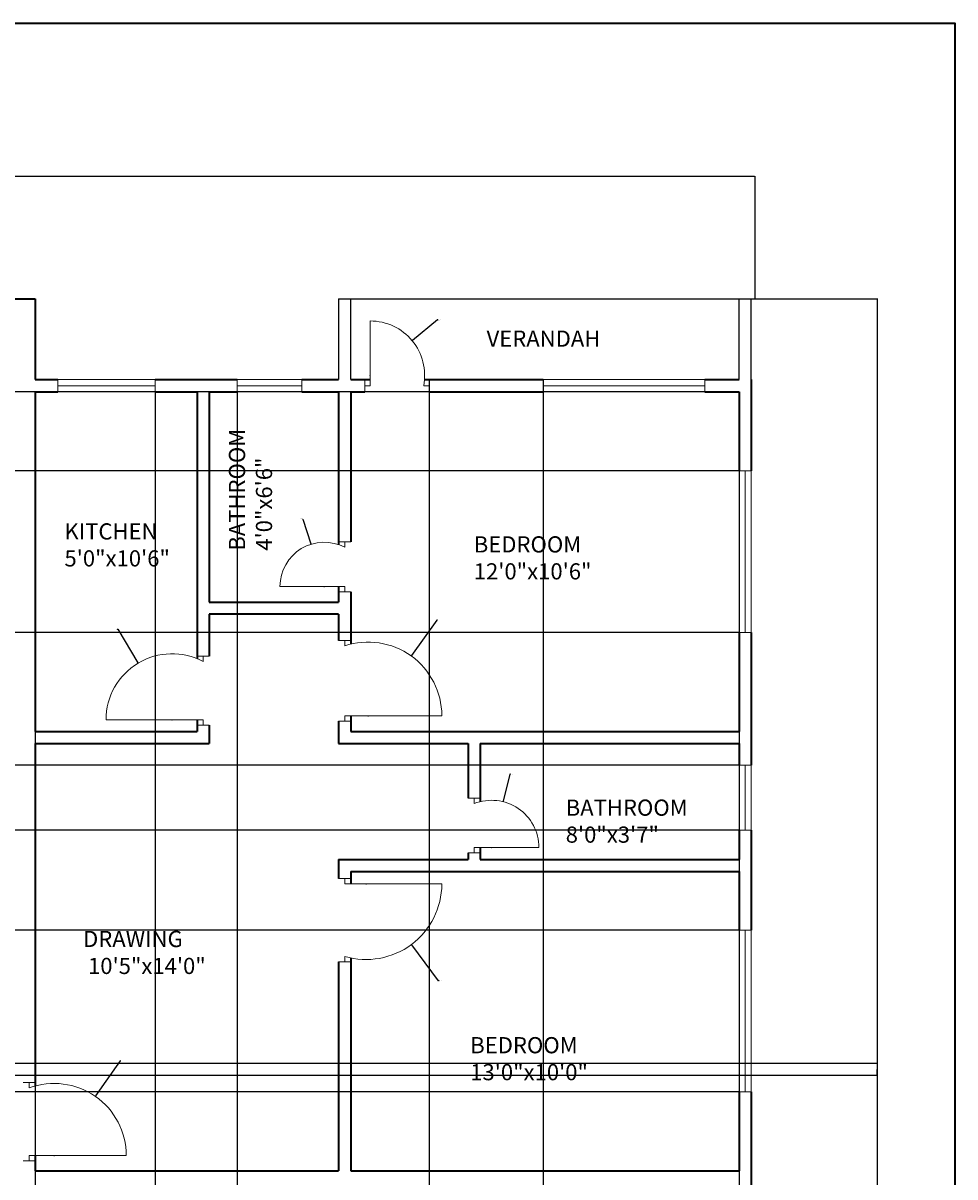
# Model space of a CAD drawing. Units: inches. Extents: x 1831 to 2867, y 1605 to 2524.
# Tile 7 of 7: x 2522 to 2867, y 2096 to 2524. Entities that reach past the tile are written whole.
import ezdxf

# ---------------------------------------------------------------- set-up
doc = ezdxf.new("R2010")
doc.units = ezdxf.units.IN
for name, color, linetype, lineweight in [('A-ANNO-DIMS', 2, 'Continuous', 18), ('A-ANNO-TTLB', 7, 'Continuous', 35), ('A-AREA-IDEN', 7, 'Continuous', 18), ('A-DOOR', 11, 'Continuous', 18), ('A-FLOR-BALC', 7, 'Continuous', 25), ('A-GLAZ', 121, 'Continuous', 18), ('A-WALL', 7, 'Continuous', 35)]:
    doc.layers.add(name, color=color, linetype=linetype, lineweight=lineweight)
doc.styles.get("Standard").update_dxf_attribs({"font": 'arial.ttf'})
doc.dimstyles.get("Standard").update_dxf_attribs({"dimtxt": 0.18, "dimasz": 0.18, "dimexe": 0.18, "dimexo": 0.0625, "dimgap": 0.09, "dimtad": 0, "dimtih": 1, "dimtoh": 1, "dimdec": 4, "dimzin": 0, "dimdsep": 46, "dimtxsty": 'Standard', "dimcen": 0.09, "dimadec": 0, "dimazin": 0, "dimtfac": 1, "dimtdec": 4, "dimtofl": 0, "dimtmove": 0, "dimatfit": 3, "dimfxl": 1, "dimtolj": 1, "dimtzin": 0, "dimarcsym": 0})

# ---------------------------------------------------------------- blocks, each defined once
blk = doc.blocks.new('WIN-60IN')
for p, q in [((4.5, 60), (0, 60)), ((0, 60), (2.25, 60)), ((0, 0), (0, 60)), ((2.25, 60), (2.25, 0)), ((4.5, 60), (4.5, 0)), ((4.5, 0), (0, 0)), ((2.25, 0), (4.5, 0))]:
    blk.add_line(p, q)
blk = doc.blocks.new('WIN-24IN')
for p, q in [((4.5, 24), (0, 24)), ((0, 24), (2.25, 24)), ((0, 0), (0, 24)), ((2.25, 24), (2.25, 0)), ((4.5, 0), (4.5, 24)), ((4.5, 0), (0, 0)), ((2.25, 0), (4.5, 0))]:
    blk.add_line(p, q)
blk = doc.blocks.new('DOOR-LEAF-36IN')
for p, q in [((0, 2), (4.5, 2)), ((4.5, 2), (2.25, 2)), ((2.25, 2), (2.25, 0)), ((2.25, 0), (38.25, 0))]:
    blk.add_line(p, q)
blk = doc.blocks.new('DOOR-LEAF-36IN-ALT')
for p, q in [((36, 2), (0, 2)), ((33.75, 0), (38.25, 0)), ((36, 0), (36, 2)), ((38.25, 0), (36, 0))]:
    blk.add_line(p, q)
blk = doc.blocks.new('DOOR-LEAF-24IN')
for p, q in [((2.25, 0), (2.25, 2)), ((2.25, 2), (26.25, 2)), ((0, 0), (4.5, 0)), ((4.5, 0), (2.25, 0))]:
    blk.add_line(p, q)
blk = doc.blocks.new('DOOR-LEAF-24IN-ALT')
for p, q in [((24, 2), (0, 2)), ((21.75, 0), (26.25, 0)), ((24, 0), (24, 2)), ((26.25, 0), (24, 0))]:
    blk.add_line(p, q)
blk = doc.blocks.new('DOOR-STRIKE-JAMB')
for p, q in [((0, 0), (4.5, 0)), ((2.25, 0), (2.25, 2)), ((4.5, 0), (2.25, 0))]:
    blk.add_line(p, q)
blk = doc.blocks.new('*D22')
at = {"layer": 'A-ANNO-DIMS', "color": 0, "lineweight": -2, "transparency": 16777216}
for p, q in [((1890.05, 2218.24), (1890.05, 2467.15)), ((1890.23, 2466.97), (2341.22, 2466.97)), ((2792.79, 2466.97), (2341.8, 2466.97)), ((2792.97, 2421.74), (2792.97, 2467.15))]:
    blk.add_line(p, q, dxfattribs=at)
at = {"layer": 'A-ANNO-DIMS', "color": 0, "transparency": 16777216}
for points in [[(1890.23, 2467), (1890.23, 2466.94), (1890.05, 2466.97)], [(2792.79, 2467), (2792.79, 2466.94), (2792.97, 2466.97)]]:
    blk.add_solid(points, dxfattribs=at)
at = {"layer": 'Defpoints', "color": 0, "transparency": 16777216}
for p in [(2792.97, 2466.97), (2792.97, 2421.67), (1890.05, 2218.17)]:
    blk.add_point(p, dxfattribs=at)
at = {"layer": 'A-ANNO-DIMS', "color": 0, "transparency": 16777216, "insert": (2341.51, 2466.97), "char_height": 0.18, "attachment_point": 5}
blk.add_mtext('\\A1;903', dxfattribs=at)
blk = doc.blocks.new('*D23')
at = {"layer": 'A-ANNO-DIMS', "color": 0, "lineweight": -2, "transparency": 16777216}
for p, q in [((2791.61, 2421.67), (2838.45, 2421.67)), ((2838.27, 2421.49), (2838.27, 2091.61)), ((2838.27, 1761.35), (2838.27, 2091.24)), ((2791.61, 1761.17), (2838.45, 1761.17))]:
    blk.add_line(p, q, dxfattribs=at)
at = {"layer": 'A-ANNO-DIMS', "color": 0, "transparency": 16777216}
for points in [[(2838.24, 2421.49), (2838.3, 2421.49), (2838.27, 2421.67)], [(2838.24, 1761.35), (2838.3, 1761.35), (2838.27, 1761.17)]]:
    blk.add_solid(points, dxfattribs=at)
at = {"layer": 'Defpoints', "color": 0, "transparency": 16777216}
for p in [(2791.55, 2421.67), (2838.27, 2421.67), (2791.55, 1761.17)]:
    blk.add_point(p, dxfattribs=at)
at = {"layer": 'A-ANNO-DIMS', "color": 0, "transparency": 16777216, "insert": (2838.27, 2091.42), "char_height": 0.18, "attachment_point": 5}
blk.add_mtext('\\A1;660.5', dxfattribs=at)
blk = doc.blocks.new('*D45')
at = {"layer": 'A-ANNO-DIMS', "color": 0, "lineweight": -2, "transparency": 16777216}
for p, q in [((2526.05, 2387.11), (2526.05, 1715.69)), ((2570.49, 2387.11), (2570.49, 1715.69)), ((2526.23, 1715.87), (2547.87, 1715.87)), ((2570.31, 1715.87), (2548.67, 1715.87))]:
    blk.add_line(p, q, dxfattribs=at)
at = {"layer": 'A-ANNO-DIMS', "color": 0, "transparency": 16777216}
for points in [[(2526.23, 1715.9), (2526.23, 1715.84), (2526.05, 1715.87)], [(2570.31, 1715.9), (2570.31, 1715.84), (2570.49, 1715.87)]]:
    blk.add_solid(points, dxfattribs=at)
at = {"layer": 'Defpoints', "color": 0, "transparency": 16777216}
for p in [(2526.05, 2387.17), (2570.49, 2387.17), (2570.49, 1715.87)]:
    blk.add_point(p, dxfattribs=at)
at = {"layer": 'A-ANNO-DIMS', "color": 0, "transparency": 16777216, "insert": (2548.27, 1715.87), "char_height": 0.18, "attachment_point": 5}
blk.add_mtext('\\A1;44.44', dxfattribs=at)
blk = doc.blocks.new('*D46')
at = {"layer": 'A-ANNO-DIMS', "color": 0, "lineweight": -2, "transparency": 16777216}
for p, q in [((2570.49, 2387.11), (2570.49, 1715.69)), ((2600.95, 2387.11), (2600.95, 1715.69)), ((2570.67, 1715.87), (2585.26, 1715.87)), ((2600.77, 1715.87), (2586.18, 1715.87))]:
    blk.add_line(p, q, dxfattribs=at)
at = {"layer": 'A-ANNO-DIMS', "color": 0, "transparency": 16777216}
for points in [[(2570.67, 1715.9), (2570.67, 1715.84), (2570.49, 1715.87)], [(2600.77, 1715.9), (2600.77, 1715.84), (2600.95, 1715.87)]]:
    blk.add_solid(points, dxfattribs=at)
at = {"layer": 'Defpoints', "color": 0, "transparency": 16777216}
for p in [(2570.49, 2387.17), (2600.95, 2387.17), (2600.95, 1715.87)]:
    blk.add_point(p, dxfattribs=at)
at = {"layer": 'A-ANNO-DIMS', "color": 0, "transparency": 16777216, "insert": (2585.72, 1715.87), "char_height": 0.18, "attachment_point": 5}
blk.add_mtext('\\A1;30.464', dxfattribs=at)
blk = doc.blocks.new('*D47')
at = {"layer": 'A-ANNO-DIMS', "color": 0, "lineweight": -2, "transparency": 16777216}
for p, q in [((2672.08, 2391.61), (2672.08, 1715.69)), ((2714.35, 2391.61), (2714.35, 1715.69)), ((2672.26, 1715.87), (2692.75, 1715.87)), ((2714.17, 1715.87), (2693.68, 1715.87))]:
    blk.add_line(p, q, dxfattribs=at)
at = {"layer": 'A-ANNO-DIMS', "color": 0, "transparency": 16777216}
for points in [[(2672.26, 1715.9), (2672.26, 1715.84), (2672.08, 1715.87)], [(2714.17, 1715.9), (2714.17, 1715.84), (2714.35, 1715.87)]]:
    blk.add_solid(points, dxfattribs=at)
at = {"layer": 'Defpoints', "color": 0, "transparency": 16777216}
for p in [(2672.08, 2391.67), (2714.35, 2391.67), (2714.35, 1715.87)]:
    blk.add_point(p, dxfattribs=at)
at = {"layer": 'A-ANNO-DIMS', "color": 0, "transparency": 16777216, "insert": (2693.22, 1715.87), "char_height": 0.18, "attachment_point": 5}
blk.add_mtext('\\A1;42.266', dxfattribs=at)
blk = doc.blocks.new('*D48')
at = {"layer": 'A-ANNO-DIMS', "color": 0, "lineweight": -2, "transparency": 16777216}
for p, q in [((2714.35, 2387.11), (2714.35, 1715.69)), ((2787.05, 2387.11), (2787.05, 1715.69)), ((2714.53, 1715.87), (2750.38, 1715.87)), ((2786.87, 1715.87), (2751.02, 1715.87))]:
    blk.add_line(p, q, dxfattribs=at)
at = {"layer": 'A-ANNO-DIMS', "color": 0, "transparency": 16777216}
for points in [[(2714.53, 1715.9), (2714.53, 1715.84), (2714.35, 1715.87)], [(2786.87, 1715.9), (2786.87, 1715.84), (2787.05, 1715.87)]]:
    blk.add_solid(points, dxfattribs=at)
at = {"layer": 'Defpoints', "color": 0, "transparency": 16777216}
for p in [(2714.35, 2387.17), (2787.05, 2387.17), (2787.05, 1715.87)]:
    blk.add_point(p, dxfattribs=at)
at = {"layer": 'A-ANNO-DIMS', "color": 0, "transparency": 16777216, "insert": (2750.7, 1715.87), "char_height": 0.18, "attachment_point": 5}
blk.add_mtext('\\A1;72.7', dxfattribs=at)
blk = doc.blocks.new('*D49')
at = {"layer": 'A-ANNO-DIMS', "color": 0, "lineweight": -2, "transparency": 16777216}
for p, q in [((2786.99, 2387.17), (1844.57, 2387.17)), ((1844.75, 2386.99), (1844.75, 2372.7)), ((1844.75, 2358.05), (1844.75, 2372.34)), ((2786.99, 2357.87), (1844.57, 2357.87))]:
    blk.add_line(p, q, dxfattribs=at)
at = {"layer": 'A-ANNO-DIMS', "color": 0, "transparency": 16777216}
for points in [[(1844.72, 2386.99), (1844.78, 2386.99), (1844.75, 2387.17)], [(1844.72, 2358.05), (1844.78, 2358.05), (1844.75, 2357.87)]]:
    blk.add_solid(points, dxfattribs=at)
at = {"layer": 'Defpoints', "color": 0, "transparency": 16777216}
for p in [(2787.05, 2387.17), (1844.75, 2357.87), (2787.05, 2357.87)]:
    blk.add_point(p, dxfattribs=at)
at = {"layer": 'A-ANNO-DIMS', "color": 0, "transparency": 16777216, "insert": (1844.75, 2372.52), "char_height": 0.18, "attachment_point": 5}
blk.add_mtext('\\A1;29.31', dxfattribs=at)
blk = doc.blocks.new('*D50')
at = {"layer": 'A-ANNO-DIMS', "color": 0, "lineweight": -2, "transparency": 16777216}
for p, q in [((2786.99, 2297.87), (1844.57, 2297.87)), ((1844.75, 2297.69), (1844.75, 2273.42)), ((1844.75, 2248.78), (1844.75, 2273.05)), ((2786.99, 2248.6), (1844.57, 2248.6))]:
    blk.add_line(p, q, dxfattribs=at)
at = {"layer": 'A-ANNO-DIMS', "color": 0, "transparency": 16777216}
for points in [[(1844.72, 2297.69), (1844.78, 2297.69), (1844.75, 2297.87)], [(1844.72, 2248.78), (1844.78, 2248.78), (1844.75, 2248.6)]]:
    blk.add_solid(points, dxfattribs=at)
at = {"layer": 'Defpoints', "color": 0, "transparency": 16777216}
for p in [(2787.05, 2297.87), (1844.75, 2248.6), (2787.05, 2248.6)]:
    blk.add_point(p, dxfattribs=at)
at = {"layer": 'A-ANNO-DIMS', "color": 0, "transparency": 16777216, "insert": (1844.75, 2273.23), "char_height": 0.18, "attachment_point": 5}
blk.add_mtext('\\A1;49.26', dxfattribs=at)
blk = doc.blocks.new('*D51')
at = {"layer": 'A-ANNO-DIMS', "color": 0, "lineweight": -2, "transparency": 16777216}
for p, q in [((2786.99, 2224.6), (1844.57, 2224.6)), ((1844.75, 2224.42), (1844.75, 2206.21)), ((1844.75, 2187.63), (1844.75, 2205.85)), ((2786.99, 2187.45), (1844.57, 2187.45))]:
    blk.add_line(p, q, dxfattribs=at)
at = {"layer": 'A-ANNO-DIMS', "color": 0, "transparency": 16777216}
for points in [[(1844.72, 2224.42), (1844.78, 2224.42), (1844.75, 2224.6)], [(1844.72, 2187.63), (1844.78, 2187.63), (1844.75, 2187.45)]]:
    blk.add_solid(points, dxfattribs=at)
at = {"layer": 'Defpoints', "color": 0, "transparency": 16777216}
for p in [(2787.05, 2224.6), (1844.75, 2187.45), (2787.05, 2187.45)]:
    blk.add_point(p, dxfattribs=at)
at = {"layer": 'A-ANNO-DIMS', "color": 0, "transparency": 16777216, "insert": (1844.75, 2206.03), "char_height": 0.18, "attachment_point": 5}
blk.add_mtext('\\A1;37.15', dxfattribs=at)
blk = doc.blocks.new('*D52')
at = {"layer": 'A-ANNO-DIMS', "color": 0, "lineweight": -2, "transparency": 16777216}
for p, q in [((2786.99, 2127.45), (1844.57, 2127.45)), ((1844.75, 2127.27), (1844.75, 2097.76)), ((1844.75, 2067.88), (1844.75, 2097.39)), ((2786.99, 2067.7), (1844.57, 2067.7))]:
    blk.add_line(p, q, dxfattribs=at)
at = {"layer": 'A-ANNO-DIMS', "color": 0, "transparency": 16777216}
for points in [[(1844.72, 2127.27), (1844.78, 2127.27), (1844.75, 2127.45)], [(1844.72, 2067.88), (1844.78, 2067.88), (1844.75, 2067.7)]]:
    blk.add_solid(points, dxfattribs=at)
at = {"layer": 'Defpoints', "color": 0, "transparency": 16777216}
for p in [(2787.05, 2127.45), (1844.75, 2067.7), (2787.05, 2067.7)]:
    blk.add_point(p, dxfattribs=at)
at = {"layer": 'A-ANNO-DIMS', "color": 0, "transparency": 16777216, "insert": (1844.75, 2097.57), "char_height": 0.18, "attachment_point": 5}
blk.add_mtext('\\A1;59.76', dxfattribs=at)
blk = doc.blocks.new('*D64')
at = {"layer": 'A-ANNO-DIMS', "color": 0, "lineweight": -2, "transparency": 16777216}
for p, q in [((2172.11, 2138.17), (2838.45, 2138.17)), ((2838.27, 2137.99), (2838.27, 2136.11)), ((2838.27, 2133.85), (2838.27, 2135.74)), ((2172.11, 2133.67), (2838.45, 2133.67))]:
    blk.add_line(p, q, dxfattribs=at)
at = {"layer": 'A-ANNO-DIMS', "color": 0, "transparency": 16777216}
for points in [[(2838.24, 2137.99), (2838.3, 2137.99), (2838.27, 2138.17)], [(2838.24, 2133.85), (2838.3, 2133.85), (2838.27, 2133.67)]]:
    blk.add_solid(points, dxfattribs=at)
at = {"layer": 'Defpoints', "color": 0, "transparency": 16777216}
for p in [(2172.05, 2138.17), (2172.05, 2133.67), (2838.27, 2133.67)]:
    blk.add_point(p, dxfattribs=at)
at = {"layer": 'A-ANNO-DIMS', "color": 0, "transparency": 16777216, "insert": (2838.27, 2135.92), "char_height": 0.18, "attachment_point": 5}
blk.add_mtext('\\A1;4.5', dxfattribs=at)
blk = doc.blocks.new('*D72')
at = {"layer": 'A-ANNO-DIMS', "color": 0, "lineweight": -2, "transparency": 16777216}
for p, q in [((2648.66, 2204.61), (2648.84, 2204.61)), ((2648.75, 2204.52), (2648.75, 2204.7)), ((2675.61, 2168.66), (2665.65, 2182)), ((2675.79, 2168.66), (2675.61, 2168.66))]:
    blk.add_line(p, q, dxfattribs=at)
at = {"layer": 'A-ANNO-DIMS', "color": 0, "transparency": 16777216}
blk.add_solid([(2665.67, 2182.02), (2665.62, 2181.98), (2665.54, 2182.14)], dxfattribs=at)
at = {"layer": 'Defpoints', "color": 0, "transparency": 16777216}
for p in [(2648.75, 2204.61), (2665.54, 2182.14)]:
    blk.add_point(p, dxfattribs=at)
at = {"layer": 'A-ANNO-DIMS', "color": 0, "transparency": 16777216, "insert": (2676.34, 2168.66), "char_height": 0.18, "attachment_point": 5}
blk.add_mtext('\\A1;R28.047', dxfattribs=at)
blk = doc.blocks.new('*D78')
at = {"layer": 'A-ANNO-DIMS', "color": 0, "lineweight": -2, "transparency": 16777216}
for p, q in [((2674.99, 2302.47), (2665.54, 2289.32)), ((2675.17, 2302.47), (2674.99, 2302.47)), ((2649.41, 2267.01), (2649.59, 2267.01)), ((2649.5, 2266.92), (2649.5, 2267.1))]:
    blk.add_line(p, q, dxfattribs=at)
at = {"layer": 'A-ANNO-DIMS', "color": 0, "transparency": 16777216}
blk.add_solid([(2665.52, 2289.34), (2665.56, 2289.3), (2665.43, 2289.17)], dxfattribs=at)
at = {"layer": 'Defpoints', "color": 0, "transparency": 16777216}
for p in [(2665.43, 2289.17), (2649.5, 2267.01)]:
    blk.add_point(p, dxfattribs=at)
at = {"layer": 'A-ANNO-DIMS', "color": 0, "transparency": 16777216, "insert": (2675.58, 2302.47), "char_height": 0.18, "attachment_point": 5}
blk.add_mtext('\\A1;R27.3', dxfattribs=at)
blk = doc.blocks.new('*D81')
at = {"layer": 'A-ANNO-DIMS', "color": 0, "lineweight": -2, "transparency": 16777216}
for p, q in [((2557.49, 2138.97), (2548.45, 2125.96)), ((2557.67, 2138.97), (2557.49, 2138.97)), ((2533.01, 2103.89), (2533.19, 2103.89)), ((2533.1, 2103.8), (2533.1, 2103.98))]:
    blk.add_line(p, q, dxfattribs=at)
at = {"layer": 'A-ANNO-DIMS', "color": 0, "transparency": 16777216}
blk.add_solid([(2548.42, 2125.98), (2548.47, 2125.95), (2548.34, 2125.82)], dxfattribs=at)
at = {"layer": 'Defpoints', "color": 0, "transparency": 16777216}
for p in [(2548.34, 2125.82), (2533.1, 2103.89)]:
    blk.add_point(p, dxfattribs=at)
at = {"layer": 'A-ANNO-DIMS', "color": 0, "transparency": 16777216, "insert": (2558.08, 2138.97), "char_height": 0.18, "attachment_point": 5}
blk.add_mtext('\\A1;R26.7', dxfattribs=at)
blk = doc.blocks.new('*D84')
at = {"layer": 'A-ANNO-DIMS', "color": 0, "lineweight": -2, "transparency": 16777216}
for p, q in [((2556.45, 2299.09), (2556.63, 2299.09)), ((2556.63, 2299.09), (2564.09, 2286.65)), ((2576.69, 2265.51), (2576.87, 2265.51)), ((2576.78, 2265.42), (2576.78, 2265.6))]:
    blk.add_line(p, q, dxfattribs=at)
at = {"layer": 'A-ANNO-DIMS', "color": 0, "transparency": 16777216}
blk.add_solid([(2564.12, 2286.67), (2564.07, 2286.64), (2564.19, 2286.5)], dxfattribs=at)
at = {"layer": 'Defpoints', "color": 0, "transparency": 16777216}
for p in [(2564.19, 2286.5), (2576.78, 2265.51)]:
    blk.add_point(p, dxfattribs=at)
at = {"layer": 'A-ANNO-DIMS', "color": 0, "transparency": 16777216, "insert": (2555.97, 2299.09), "char_height": 0.18, "attachment_point": 5}
blk.add_mtext('\\A1;R24.48', dxfattribs=at)
blk = doc.blocks.new('*D85')
at = {"layer": 'A-ANNO-DIMS', "color": 0, "lineweight": -2, "transparency": 16777216}
for p, q in [((2675.17, 2413.8), (2665.97, 2406.21)), ((2675.35, 2413.8), (2675.17, 2413.8)), ((2650.18, 2393.25), (2650.36, 2393.25)), ((2650.27, 2393.16), (2650.27, 2393.34))]:
    blk.add_line(p, q, dxfattribs=at)
at = {"layer": 'A-ANNO-DIMS', "color": 0, "transparency": 16777216}
blk.add_solid([(2665.95, 2406.23), (2665.99, 2406.18), (2665.83, 2406.09)], dxfattribs=at)
at = {"layer": 'Defpoints', "color": 0, "transparency": 16777216}
for p in [(2665.83, 2406.09), (2650.27, 2393.25)]:
    blk.add_point(p, dxfattribs=at)
at = {"layer": 'A-ANNO-DIMS', "color": 0, "transparency": 16777216, "insert": (2675.83, 2413.8), "char_height": 0.18, "attachment_point": 5}
blk.add_mtext('\\A1;R20.18', dxfattribs=at)
blk = doc.blocks.new('*D102')
at = {"layer": 'A-ANNO-DIMS', "color": 0, "lineweight": -2, "transparency": 16777216}
for p, q in [((2625.09, 2339.95), (2625.27, 2339.95)), ((2625.27, 2339.95), (2628.18, 2330.76)), ((2633.08, 2314.98), (2633.26, 2314.98)), ((2633.17, 2314.89), (2633.17, 2315.07))]:
    blk.add_line(p, q, dxfattribs=at)
at = {"layer": 'A-ANNO-DIMS', "color": 0, "transparency": 16777216}
blk.add_solid([(2628.21, 2330.77), (2628.15, 2330.75), (2628.23, 2330.59)], dxfattribs=at)
at = {"layer": 'Defpoints', "color": 0, "transparency": 16777216}
for p in [(2628.23, 2330.59), (2633.17, 2314.98)]:
    blk.add_point(p, dxfattribs=at)
at = {"layer": 'A-ANNO-DIMS', "color": 0, "transparency": 16777216, "insert": (2624.61, 2339.95), "char_height": 0.18, "attachment_point": 5}
blk.add_mtext('\\A1;R16.37', dxfattribs=at)
blk = doc.blocks.new('*D103')
at = {"layer": 'A-ANNO-DIMS', "color": 0, "lineweight": -2, "transparency": 16777216}
for p, q in [((2702.07, 2245.31), (2699.57, 2235.28)), ((2702.25, 2245.31), (2702.07, 2245.31)), ((2695.2, 2218.11), (2695.38, 2218.11)), ((2695.29, 2218.02), (2695.29, 2218.2))]:
    blk.add_line(p, q, dxfattribs=at)
at = {"layer": 'A-ANNO-DIMS', "color": 0, "transparency": 16777216}
blk.add_solid([(2699.54, 2235.29), (2699.6, 2235.28), (2699.53, 2235.11)], dxfattribs=at)
at = {"layer": 'Defpoints', "color": 0, "transparency": 16777216}
for p in [(2699.53, 2235.11), (2695.29, 2218.11)]:
    blk.add_point(p, dxfattribs=at)
at = {"layer": 'A-ANNO-DIMS', "color": 0, "transparency": 16777216, "insert": (2702.8, 2245.31), "char_height": 0.18, "attachment_point": 5}
blk.add_mtext('\\A1;R17.516', dxfattribs=at)

msp = doc.modelspace()

# ---------------------------------------------------------------- linework, layer by layer
at = {"layer": 'A-ANNO-TTLB'}
msp.add_lwpolyline([(1831.1248, 2523.9204), (2867.0416, 2523.9204), (2867.0416, 1605.0781), (1831.1248, 1605.0781)], close=True, dxfattribs=at)
at = {"layer": 'A-DOOR'}
for centre, radius, start, end in [((2650.2704, 2393.2454), 20.1784, 349.0827, 90), ((2633.1702, 2314.9792), 16.3692, 62.214167, 180), ((2649.5026, 2267.005), 27.2984, 0, 108.587864), ((2576.7798, 2265.5082), 24.4788, 61.922764, 180), ((2695.2854, 2218.1146), 17.5156, 360, 111.728297), ((2648.7544, 2204.6131), 28.0466, 253.526069, 0), ((2533.1, 2103.8924), 26.701, 360, 110.38115)]:
    msp.add_arc(centre, radius, start, end, dxfattribs=at)
at = {"layer": 'A-FLOR-BALC'}
for p, q in [((2638.551, 2421.6738), (2638.551, 2391.6738)), ((2638.551, 2421.6738), (2792.9663, 2421.6738)), ((2643.051, 2391.6738), (2643.051, 2421.6738)), ((2787.051, 2391.6738), (2787.051, 2421.6738)), ((2791.551, 2391.6738), (2791.551, 2421.6738))]:
    msp.add_line(p, q, dxfattribs=at)
at = {"layer": 'A-GLAZ'}
for p, q in [((2534.4894, 2391.6738), (2534.4894, 2387.1738)), ((2570.4894, 2391.6738), (2534.4894, 2391.6738)), ((2534.4894, 2387.1738), (2534.4894, 2389.4238)), ((2534.4894, 2389.4238), (2570.4894, 2389.4238)), ((2570.4894, 2389.4238), (2570.4894, 2391.6738)), ((2570.4894, 2389.4238), (2570.4894, 2389.4238)), ((2570.4894, 2389.4238), (2570.4894, 2387.1738)), ((2624.9537, 2391.6738), (2600.433, 2391.6738)), ((2600.9537, 2387.1738), (2600.9537, 2391.6738)), ((2600.9537, 2391.6738), (2600.9537, 2389.4238)), ((2600.9537, 2389.4238), (2624.9537, 2389.4238)), ((2624.9537, 2389.4238), (2624.9537, 2391.6738)), ((2624.9537, 2391.6738), (2624.9537, 2387.1738)), ((2533.9102, 2387.1738), (2570.4894, 2387.1738)), ((2600.9537, 2387.1738), (2624.9537, 2387.1738)), ((2787.051, 2127.452), (2787.051, 2127.452))]:
    msp.add_line(p, q, dxfattribs=at)
at = {"layer": 'A-WALL'}
for p, q in [((2485.4746, 2421.6738), (2526.051, 2421.6738)), ((2526.051, 2421.6738), (2526.051, 2391.6738)), ((2526.051, 2391.6738), (2534.4894, 2391.6738)), ((2570.4894, 2391.6738), (2600.9537, 2391.6738)), ((2624.9537, 2391.6738), (2638.551, 2391.6738)), ((2643.051, 2391.6738), (2650.2704, 2391.6738)), ((2670.3874, 2391.6738), (2714.3491, 2391.6738)), ((2774.3491, 2391.6738), (2787.051, 2391.6738)), ((2791.551, 2391.6738), (2791.551, 2357.8655)), ((2526.051, 2387.1738), (2526.051, 2261.1738)), ((2526.051, 2387.1738), (2534.4894, 2387.1738)), ((2526.051, 2387.1738), (2526.051, 2261.1738)), ((2570.4894, 2387.1738), (2586.051, 2387.1738)), ((2586.051, 2387.1738), (2586.051, 2288.1634)), ((2590.551, 2387.1738), (2590.551, 2309.1738)), ((2590.551, 2387.1738), (2600.9537, 2387.1738)), ((2590.551, 2387.1738), (2590.551, 2309.1738)), ((2624.9537, 2387.1738), (2638.551, 2387.1738)), ((2638.551, 2387.1738), (2638.551, 2330.4387)), ((2643.051, 2387.1738), (2643.051, 2331.4609)), ((2643.051, 2387.1738), (2648.2704, 2387.1738)), ((2672.0835, 2387.1738), (2714.3491, 2387.1738)), ((2774.3491, 2387.1738), (2787.051, 2387.1738)), ((2787.051, 2387.1738), (2787.051, 2357.8655)), ((2638.551, 2314.9792), (2638.551, 2309.1738)), ((2643.051, 2312.9792), (2643.051, 2293.5301)), ((2590.551, 2309.1738), (2638.551, 2309.1738)), ((2638.551, 2304.6738), (2590.551, 2304.6738)), ((2590.551, 2304.6738), (2590.551, 2289.1062)), ((2638.551, 2304.6738), (2638.551, 2294.8794)), ((2787.051, 2297.8655), (2787.051, 2261.1738)), ((2791.551, 2297.8655), (2791.551, 2248.6027)), ((2586.051, 2265.5082), (2586.051, 2261.1738)), ((2638.551, 2265.005), (2638.551, 2261.1738)), ((2643.051, 2267.005), (2643.051, 2261.1738)), ((2526.051, 2261.1738), (2586.051, 2261.1738)), ((2590.551, 2263.5082), (2590.551, 2261.1738)), ((2590.551, 2261.1738), (2590.551, 2256.6738)), ((2638.551, 2261.1738), (2638.551, 2256.6738)), ((2643.051, 2261.1738), (2787.051, 2261.1738)), ((2526.051, 2256.6738), (2526.051, 2129.6462)), ((2526.051, 2256.6738), (2590.551, 2256.6738)), ((2638.551, 2256.6738), (2686.551, 2256.6738)), ((2686.551, 2256.6738), (2686.551, 2236.3857)), ((2691.051, 2256.6738), (2691.051, 2235.1107)), ((2691.051, 2256.6738), (2787.051, 2256.6738)), ((2787.051, 2256.6738), (2787.051, 2248.6027)), ((2787.051, 2224.6027), (2787.051, 2213.6738)), ((2791.551, 2224.6027), (2791.551, 2187.452)), ((2691.051, 2218.1146), (2691.051, 2213.6738)), ((2638.551, 2213.6738), (2638.551, 2206.6131)), ((2638.551, 2213.6738), (2686.551, 2213.6738)), ((2686.551, 2216.1146), (2686.551, 2213.6738)), ((2691.051, 2213.6738), (2787.051, 2213.6738)), ((2643.051, 2209.1738), (2643.051, 2204.6131)), ((2643.051, 2209.1738), (2787.051, 2209.1738)), ((2787.051, 2209.1738), (2787.051, 2187.452)), ((2638.551, 2175.7178), (2638.551, 2098.1738)), ((2643.051, 2177.1525), (2643.051, 2098.1738)), ((2787.051, 2127.452), (2787.051, 2098.1738)), ((2791.551, 2127.452), (2791.551, 2067.6955)), ((2526.051, 2103.8924), (2526.051, 2098.1738)), ((2526.051, 2098.1738), (2638.551, 2098.1738)), ((2643.051, 2098.1738), (2787.051, 2098.1738))]:
    msp.add_line(p, q, dxfattribs=at)

# ---------------------------------------------------------------- block references
at = {"layer": 'A-DOOR', "rotation": 269.9999999999989}
msp.add_blockref('DOOR-LEAF-24IN-ALT', (2648.2704, 2413.4238), dxfattribs=at)
at = {"layer": 'A-DOOR', "extrusion": (0, 0, -1), "zscale": -1}
for name, p, rotation in [('DOOR-STRIKE-JAMB', (-2672.0835, 2391.6738), 270.0000000000085), ('DOOR-STRIKE-JAMB', (-2638.551, 2331.4609), 180), ('DOOR-STRIKE-JAMB', (-2638.551, 2294.8794), 180), ('DOOR-STRIKE-JAMB', (-2586.051, 2289.1062), 180), ('DOOR-LEAF-36IN', (-2638.551, 2267.005), 180), ('DOOR-STRIKE-JAMB', (-2686.551, 2236.3857), 180), ('DOOR-STRIKE-JAMB', (-2521.551, 2130.9218), 180)]:
    msp.add_blockref(name, p, dxfattribs=dict(at, rotation=rotation))
at = {"layer": 'A-DOOR'}
for name, p in [('DOOR-LEAF-24IN-ALT', (2616.801, 2312.9792)), ('DOOR-LEAF-36IN-ALT', (2552.301, 2263.5082)), ('DOOR-LEAF-24IN', (2686.551, 2216.1146)), ('DOOR-LEAF-36IN', (2638.551, 2204.6131)), ('DOOR-STRIKE-JAMB', (2638.551, 2175.7178))]:
    msp.add_blockref(name, p, dxfattribs=at)
at = {"layer": 'A-DOOR', "extrusion": (0, 0, -1), "zscale": -1}
msp.add_blockref('DOOR-LEAF-36IN-ALT', (-2559.801, 2101.8924), dxfattribs=at)
at = {"layer": 'A-GLAZ', "extrusion": (0, 0, -1), "zscale": -1}
for name, p, rotation in [('WIN-60IN', (-2774.3491, 2391.6738), 269.9999999999988), ('WIN-60IN', (-2787.051, 2357.8655), 180), ('WIN-24IN', (-2787.051, 2248.6027), 180)]:
    msp.add_blockref(name, p, dxfattribs=dict(at, rotation=rotation))
at = {"layer": 'A-GLAZ', "rotation": 180}
msp.add_blockref('WIN-60IN', (2791.551, 2187.452), dxfattribs=at)

# ---------------------------------------------------------------- texts
at = {"layer": 'A-AREA-IDEN', "char_height": 6, "attachment_point": 1}
for s, width, insert in [('VERANDAH', 121.894867, (2693.3967, 2409.8774)), ('KITCHEN\\P5\'0"x10\'6"', 124.661971, (2536.8932, 2338.366)), ('BEDROOM\\P12\'0"x10\'6"', 141.265394, (2688.6535, 2333.5483)), ('BATHROOM\\P8\'0"x3\'7"', 96.524155, (2722.743, 2235.8949)), ('DRAWING\\P 10\'5"x14\'0"', 177.829253, (2543.7965, 2187.1906)), ('BEDROOM\\P13\'0"x10\'0"', 168.557957, (2687.3349, 2147.7855))]:
    msp.add_mtext_dynamic_manual_height_columns(s, width=width, gutter_width=12.5, heights=[0], dxfattribs=dict(at, insert=insert))
at = {"layer": 'A-AREA-IDEN', "insert": (2597.8685, 2328.2067), "char_height": 6, "attachment_point": 1, "rotation": 90}
msp.add_mtext_dynamic_manual_height_columns('BATHROOM\\P4\'0"x6\'6"', width=75.922121, gutter_width=12.5, heights=[0], dxfattribs=at)

# ---------------------------------------------------------------- dimensions: what is measured, and where the dimension line sits
at = {"layer": 'A-ANNO-DIMS'}
for base, p1, p2, override, picture, middle in [((2792.9663, 2466.9738), (1890.051, 2218.1738), (2792.9663, 2421.6738), {"dimdec": 0, "dimlfac": 1, "dimrnd": 0, "dimzin": 0, "dimdsep": 46, "dimlunit": 2}, '*D22', (2341.5086, 2466.9738)), ((2714.3491, 1715.8738), (2672.0835, 2391.6738), (2714.3491, 2391.6738), {"dimdec": 3, "dimlfac": 1, "dimrnd": 0, "dimzin": 0, "dimdsep": 46, "dimlunit": 2}, '*D47', (2693.2163, 1715.8738)), ((2570.4894, 1715.8738), (2526.051, 2387.1738), (2570.4894, 2387.1738), {"dimdec": 2, "dimlfac": 1, "dimrnd": 0, "dimzin": 0, "dimdsep": 46, "dimlunit": 2}, '*D45', (2548.2702, 1715.8738)), ((2600.9537, 1715.8738), (2570.4894, 2387.1738), (2600.9537, 2387.1738), {"dimdec": 3, "dimlfac": 1, "dimrnd": 0, "dimzin": 0, "dimdsep": 46, "dimlunit": 2}, '*D46', (2585.7216, 1715.8738)), ((2787.051, 1715.8738), (2714.3491, 2387.1738), (2787.051, 2387.1738), {"dimdec": 1, "dimlfac": 1, "dimrnd": 0, "dimzin": 0, "dimdsep": 46, "dimlunit": 2}, '*D48', (2750.7001, 1715.8738))]:
    dim = msp.add_linear_dim(base=base, p1=p1, p2=p2, dimstyle='Standard', override=override, dxfattribs=at)
    dim.commit()
    dim.dimension.update_dxf_attribs({"geometry": picture, "text_midpoint": middle})
for base, p1, p2, override, picture, middle in [((2838.2663, 2421.6738), (2791.551, 1761.1738), (2791.551, 2421.6738), {"dimdec": 1, "dimlfac": 1, "dimrnd": 0, "dimzin": 0, "dimdsep": 46, "dimlunit": 2}, '*D23', (2838.2663, 2091.4238)), ((1844.751, 2357.8655), (2787.051, 2387.1738), (2787.051, 2357.8655), {"dimdec": 2, "dimlfac": 1, "dimrnd": 0, "dimzin": 0, "dimdsep": 46, "dimlunit": 2}, '*D49', (1844.751, 2372.5196)), ((1844.751, 2248.6027), (2787.051, 2297.8655), (2787.051, 2248.6027), {"dimdec": 2, "dimlfac": 1, "dimrnd": 0, "dimzin": 0, "dimdsep": 46, "dimlunit": 2}, '*D50', (1844.751, 2273.2341)), ((1844.751, 2187.452), (2787.051, 2224.6027), (2787.051, 2187.452), {"dimdec": 2, "dimlfac": 1, "dimrnd": 0, "dimzin": 0, "dimdsep": 46, "dimlunit": 2}, '*D51', (1844.751, 2206.0273)), ((2838.2663, 2133.6738), (2172.051, 2138.1738), (2172.051, 2133.6738), {"dimdec": 1, "dimlfac": 1, "dimrnd": 0, "dimzin": 0, "dimdsep": 46, "dimlunit": 2}, '*D64', (2838.2663, 2135.9238)), ((1844.751, 2067.6955), (2787.051, 2127.452), (2787.051, 2067.6955), {"dimdec": 2, "dimlfac": 1, "dimrnd": 0, "dimzin": 0, "dimdsep": 46, "dimlunit": 2}, '*D52', (1844.751, 2097.5738))]:
    dim = msp.add_linear_dim(base=base, p1=p1, p2=p2, angle=90, dimstyle='Standard', override=override, dxfattribs=at)
    dim.commit()
    dim.dimension.update_dxf_attribs({"geometry": picture, "text_midpoint": middle})
for center, mpoint, override, picture, middle in [((2650.2704, 2393.2454), (2665.831, 2406.092), {"dimdec": 2, "dimlfac": 1, "dimrnd": 0, "dimzin": 0, "dimdsep": 46, "dimlunit": 2}, '*D85', (2675.8273, 2413.7999)), ((2633.1702, 2314.9792), (2628.2328, 2330.586), {"dimdec": 2, "dimlfac": 1, "dimrnd": 0, "dimzin": 0, "dimdsep": 46, "dimlunit": 2}, '*D102', (2624.6105, 2339.9501)), ((2576.7798, 2265.5082), (2564.1861, 2286.4989), {"dimdec": 2, "dimlfac": 1, "dimrnd": 0, "dimzin": 0, "dimdsep": 46, "dimlunit": 2}, '*D84', (2555.9698, 2299.0933)), ((2649.5026, 2267.005), (2665.4349, 2289.1718), {"dimdec": 1, "dimlfac": 1, "dimrnd": 0, "dimzin": 0, "dimdsep": 46, "dimlunit": 2}, '*D78', (2675.5841, 2302.4719)), ((2695.2854, 2218.1146), (2699.5263, 2235.1091), {"dimdec": 3, "dimlfac": 1, "dimrnd": 0, "dimzin": 0, "dimdsep": 46, "dimlunit": 2}, '*D103', (2702.8006, 2245.3057)), ((2648.7544, 2204.6131), (2665.54, 2182.1441), {"dimdec": 3, "dimlfac": 1, "dimrnd": 0, "dimzin": 0, "dimdsep": 46, "dimlunit": 2}, '*D72', (2676.341, 2168.6627)), ((2533.1, 2103.8924), (2548.3423, 2125.8154), {"dimdec": 1, "dimlfac": 1, "dimrnd": 0, "dimzin": 0, "dimdsep": 46, "dimlunit": 2}, '*D81', (2558.0775, 2138.9692))]:
    dim = msp.add_radius_dim(center=center, mpoint=mpoint, dimstyle='Standard', override=override, dxfattribs=at)
    dim.commit()
    dim.dimension.update_dxf_attribs({"geometry": picture, "text_midpoint": middle, "dimtype": 164})

doc.saveas('drawing.dxf')
